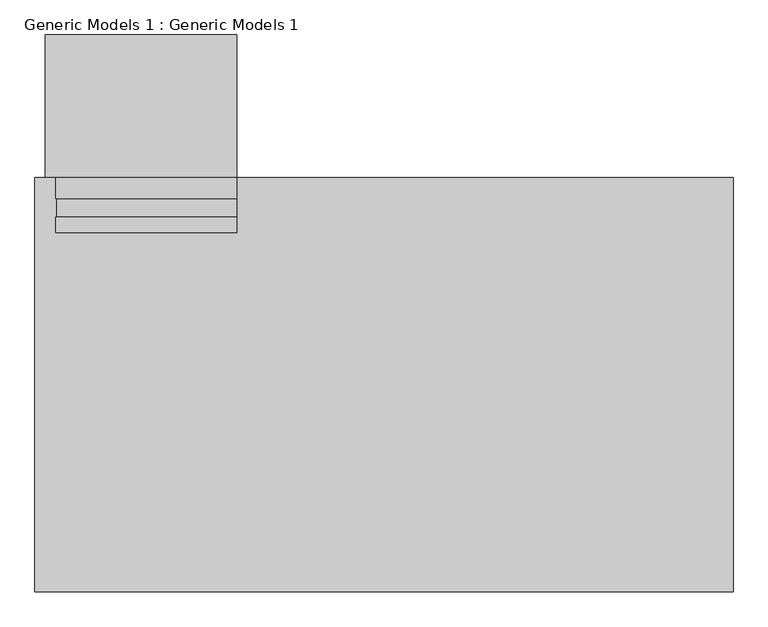
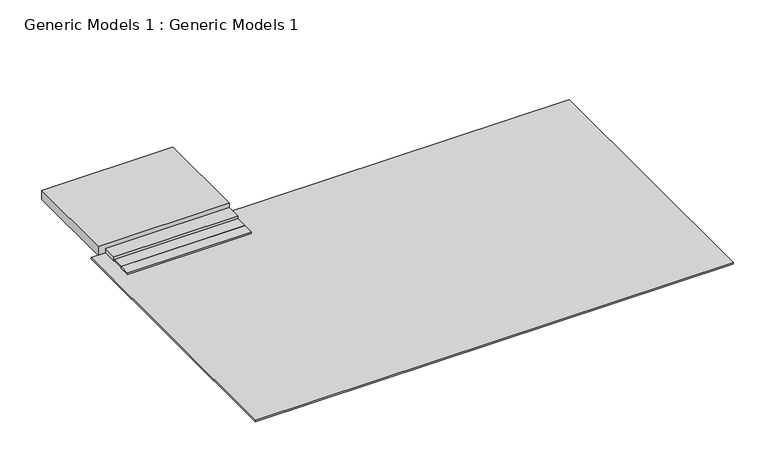
"""IFC4 building model written with IfcOpenShell, lengths in millimetres: proxy geometry, Generic Models 1 : Generic Models 1."""

from ifc_helpers import new_model, si_unit, frame, origin, origin_with_axes, place, context, project, spatial, polyline, outline, extrude, source, transform, mapped, element, save


def generic_models_1_generic_models_1_7cf849b9(model_context):
    return source(origin(), model_context, "Body", "SweptSolid", [
        extrude(outline(polyline([(-18852.414323, -14748.2931134), (-14788.414323, -14748.2931134), (-14788.414323, -15103.8931134), (-18852.414323, -15103.8931134), (-18852.414323, -14748.2931134)])), frame((0.0, 0.0, -25.4), z_axis=(0.0, 0.0, 1.0), x_axis=(1.0, 0.0, 0.0)), (0.0, 0.0, 1.0), 86.9878233),
        extrude(outline(polyline([(-14788.414323, -14748.2931134), (-18827.014323, -14748.2931134), (-18827.014323, -14341.8931134), (-14788.414323, -14341.8931134), (-14788.414323, -14748.2931134)])), origin_with_axes(), (0.0, 0.0, 1.0), 61.5878233),
        extrude(outline(polyline([(-14788.414323, -14341.8931134), (-18857.6625313, -14341.8931134), (-18857.6625313, -13854.1538163), (-14788.414323, -13854.1538163), (-14788.414323, -14341.8931134)])), origin_with_axes(), (0.0, 0.0, 1.0), 152.4),
        extrude(outline(polyline([(-3625.114323, -13864.3466243), (-3625.114323, -23188.6538163), (-19322.314323, -23188.6538163), (-19322.314323, -13864.3466243), (-3625.114323, -13864.3466243)])), frame((0.0, 0.0, -50.8), z_axis=(0.0, 0.0, 1.0), x_axis=(1.0, 0.0, 0.0)), (0.0, 0.0, 1.0), 50.8),
        extrude(outline(polyline([(-14788.414323, -10653.7538163), (-14788.414323, -13854.1538163), (-19093.714323, -13854.1538163), (-19093.714323, -10653.7538163), (-14788.414323, -10653.7538163)])), origin_with_axes(), (0.0, 0.0, 1.0), 304.8),
    ])


if __name__ == "__main__":
    model = new_model("IFC4")
    model_context = context("Model", 3, world=origin())
    ifc_project = project(units=[si_unit("LENGTHUNIT", "METRE", prefix="MILLI")], contexts=[model_context])
    site = spatial("IfcSite", under=ifc_project)
    building = spatial("IfcBuilding", under=site)
    placement = place(None, origin())
    generic_models_1_generic_models_1_shape = generic_models_1_generic_models_1_7cf849b9(model_context)
    element("IfcBuildingElementProxy", 1, Name="Generic Models 1 : Generic Models 1", ObjectType="Generic Models 1 : Generic Models 1", at=placement, inside=building, context=model_context, shape_type="MappedRepresentation", body=[
        mapped(generic_models_1_generic_models_1_shape, transform((0.0, 0.0, 0.0), x_axis=(1.0, 0.0, 0.0), y_axis=(0.0, 1.0, 0.0), z_axis=(0.0, 0.0, 1.0))),
    ])
    save(model, "model.ifc")
